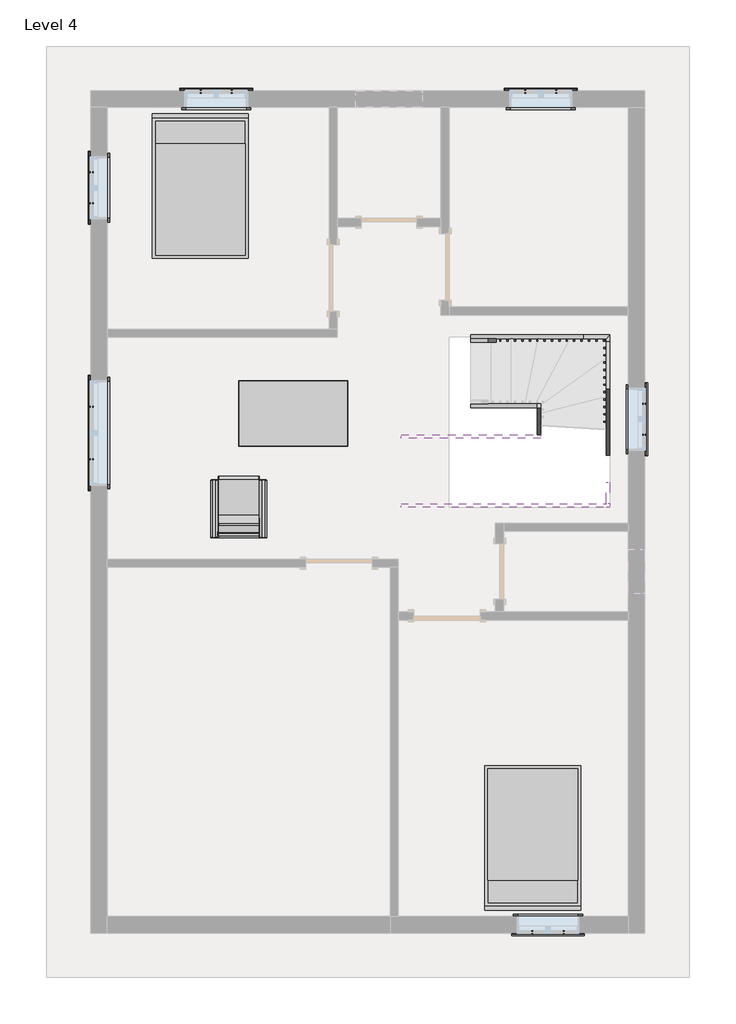
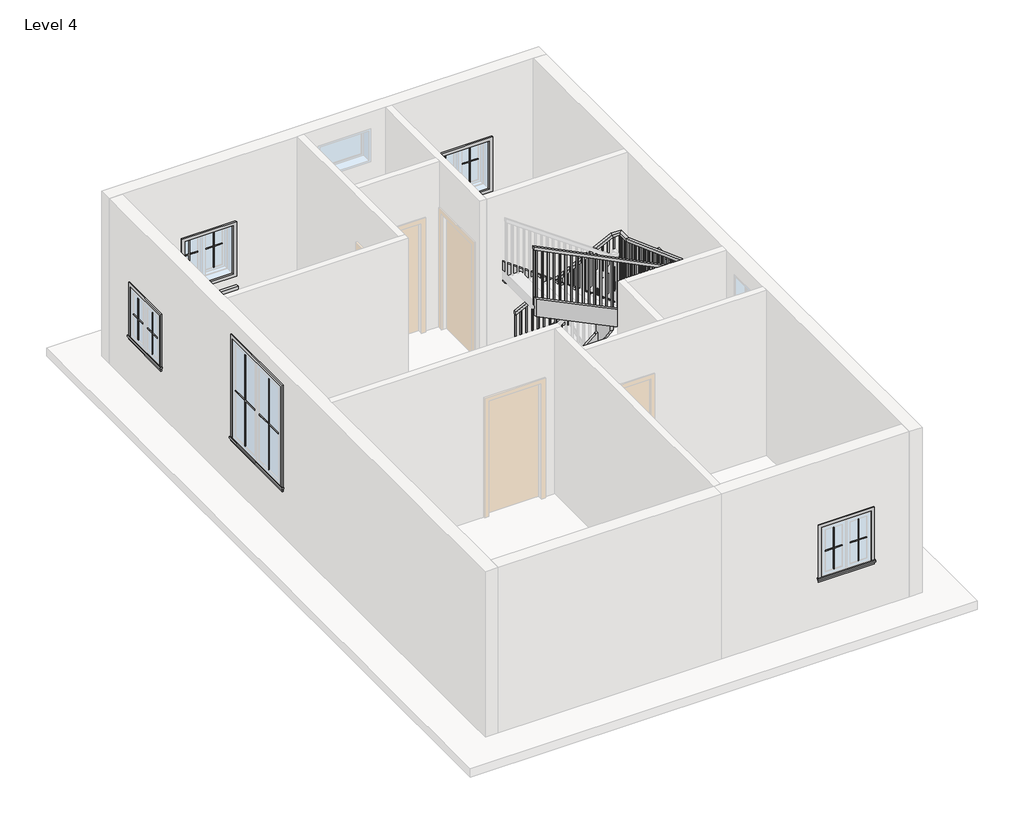
# One storey, part 2 of 2: 24 proxies, 9 members, 4 furniture elements, 1 railing.
"""IFC4 building model written with IfcOpenShell, lengths in millimetres."""

from ifc_helpers import new_model, si_unit, frame, origin, place, context, project, spatial, polyline, outline, extrude, faceted_brep, transform, mapped, element, save
from components import muntin_pattern_2x2_muntin_pattern_2x2_b3fe6957, muntin_pattern_2x2_muntin_pattern_2x2_3e0ecaf2, muntin_pattern_2x2_muntin_pattern_2x2_bff912c5, muntin_pattern_2x2_muntin_pattern_2x2_c2194282, trim_window_exterior_flat_with_sill_41619996, trim_window_exterior_flat_with_sill_e04b3088, trim_window_interior_flat_picture_frame_51c85655, trim_window_interior_flat_picture_frame_2a7685fe, furniture_f28dd14e, furniture_402a1f5e, bed_17739_bed_17739_15c61121, dining_table_14755_dining_table_14755_d89cb775

model = new_model("IFC4")

# Units and contexts
model_context = context("Model", 3, world=origin())
ifc_project = project(units=[si_unit("LENGTHUNIT", "METRE", prefix="MILLI")], contexts=[model_context])

# Site, building, storey
site = spatial("IfcSite", under=ifc_project)
building = spatial("IfcBuilding", under=site)
storey = spatial("IfcBuildingStorey", under=building, Name="Level 4", Elevation=6400.8)

# Proxies
placement = place(None, origin())
muntin_pattern_2x2_muntin_pattern_2x2_shape = muntin_pattern_2x2_muntin_pattern_2x2_b3fe6957(model_context)
element("IfcBuildingElementProxy", 1, Name="Muntin Pattern_2x2 : Muntin Pattern_2x2", ObjectType="Muntin Pattern_2x2 : Muntin Pattern_2x2", at=placement, inside=storey, context=model_context, shape_type="MappedRepresentation", body=[
    mapped(muntin_pattern_2x2_muntin_pattern_2x2_shape, transform((-3555.5290084, 6319.8685985, 7385.05), x_axis=(1.0, 0.0, 0.0), y_axis=(0.0, 1.0, 0.0), z_axis=(0.0, 0.0, 1.0))),
])
element("IfcBuildingElementProxy", 2, Name="Muntin Pattern_2x2 : Muntin Pattern_2x2", ObjectType="Muntin Pattern_2x2 : Muntin Pattern_2x2", at=placement, inside=storey, context=model_context, shape_type="MappedRepresentation", body=[
    mapped(muntin_pattern_2x2_muntin_pattern_2x2_shape, transform((1435.5709916, -5243.4814015, 7385.05), x_axis=(-1.0, 0.0, 0.0), y_axis=(0.0, -1.0, 0.0), z_axis=(0.0, 0.0, 1.0))),
])
element("IfcBuildingElementProxy", 3, Name="Muntin Pattern_2x2 : Muntin Pattern_2x2", ObjectType="Muntin Pattern_2x2 : Muntin Pattern_2x2", at=placement, inside=storey, context=model_context, shape_type="MappedRepresentation", body=[
    mapped(muntin_pattern_2x2_muntin_pattern_2x2_shape, transform((2545.2334916, 2028.8560985, 7385.05), x_axis=(0.0, -1.0, 0.0), y_axis=(1.0, 0.0, 0.0), z_axis=(0.0, 0.0, 1.0))),
])
element("IfcBuildingElementProxy", 4, Name="Muntin Pattern_2x2 : Muntin Pattern_2x2", ObjectType="Muntin Pattern_2x2 : Muntin Pattern_2x2", at=placement, inside=storey, context=model_context, shape_type="MappedRepresentation", body=[
    mapped(muntin_pattern_2x2_muntin_pattern_2x2_shape, transform((908.5209916, 6319.8685985, 7385.05), x_axis=(1.0, 0.0, 0.0), y_axis=(0.0, 1.0, 0.0), z_axis=(0.0, 0.0, 1.0))),
])
element("IfcBuildingElementProxy", 5, Name="Muntin Pattern_2x2 : Muntin Pattern_2x2", ObjectType="Muntin Pattern_2x2 : Muntin Pattern_2x2", at=placement, inside=storey, context=model_context, shape_type="MappedRepresentation", body=[
    mapped(muntin_pattern_2x2_muntin_pattern_2x2_shape, transform((-5055.7165084, 4781.5810985, 7385.05), x_axis=(0.0, 1.0, 0.0), y_axis=(-1.0, 0.0, 0.0), z_axis=(0.0, 0.0, 1.0))),
])
muntin_pattern_2x2_muntin_pattern_2x2_2_shape = muntin_pattern_2x2_muntin_pattern_2x2_3e0ecaf2(model_context)
element("IfcBuildingElementProxy", 6, Name="Muntin Pattern_2x2 : Muntin Pattern_2x2", ObjectType="Muntin Pattern_2x2 : Muntin Pattern_2x2", at=placement, inside=storey, context=model_context, shape_type="MappedRepresentation", body=[
    mapped(muntin_pattern_2x2_muntin_pattern_2x2_2_shape, transform((-3126.9040084, 6319.8685985, 7385.05), x_axis=(-1.0, 0.0, 0.0), y_axis=(0.0, -1.0, 0.0), z_axis=(0.0, 0.0, 1.0))),
])
element("IfcBuildingElementProxy", 7, Name="Muntin Pattern_2x2 : Muntin Pattern_2x2", ObjectType="Muntin Pattern_2x2 : Muntin Pattern_2x2", at=placement, inside=storey, context=model_context, shape_type="MappedRepresentation", body=[
    mapped(muntin_pattern_2x2_muntin_pattern_2x2_2_shape, transform((1006.9459916, -5243.4814015, 7385.05), x_axis=(1.0, 0.0, 0.0), y_axis=(0.0, 1.0, 0.0), z_axis=(0.0, 0.0, 1.0))),
])
element("IfcBuildingElementProxy", 8, Name="Muntin Pattern_2x2 : Muntin Pattern_2x2", ObjectType="Muntin Pattern_2x2 : Muntin Pattern_2x2", at=placement, inside=storey, context=model_context, shape_type="MappedRepresentation", body=[
    mapped(muntin_pattern_2x2_muntin_pattern_2x2_2_shape, transform((2545.2334916, 1600.2310985, 7385.05), x_axis=(0.0, 1.0, 0.0), y_axis=(-1.0, 0.0, 0.0), z_axis=(0.0, 0.0, 1.0))),
])
element("IfcBuildingElementProxy", 9, Name="Muntin Pattern_2x2 : Muntin Pattern_2x2", ObjectType="Muntin Pattern_2x2 : Muntin Pattern_2x2", at=placement, inside=storey, context=model_context, shape_type="MappedRepresentation", body=[
    mapped(muntin_pattern_2x2_muntin_pattern_2x2_2_shape, transform((1337.1459916, 6319.8685985, 7385.05), x_axis=(-1.0, 0.0, 0.0), y_axis=(0.0, -1.0, 0.0), z_axis=(0.0, 0.0, 1.0))),
])
element("IfcBuildingElementProxy", 10, Name="Muntin Pattern_2x2 : Muntin Pattern_2x2", ObjectType="Muntin Pattern_2x2 : Muntin Pattern_2x2", at=placement, inside=storey, context=model_context, shape_type="MappedRepresentation", body=[
    mapped(muntin_pattern_2x2_muntin_pattern_2x2_2_shape, transform((-5055.7165084, 5210.2060985, 7385.05), x_axis=(0.0, -1.0, 0.0), y_axis=(1.0, 0.0, 0.0), z_axis=(0.0, 0.0, 1.0))),
])
muntin_pattern_2x2_muntin_pattern_2x2_3_shape = muntin_pattern_2x2_muntin_pattern_2x2_bff912c5(model_context)
element("IfcBuildingElementProxy", 11, Name="Muntin Pattern_2x2 : Muntin Pattern_2x2", ObjectType="Muntin Pattern_2x2 : Muntin Pattern_2x2", at=placement, inside=storey, context=model_context, shape_type="MappedRepresentation", body=[
    mapped(muntin_pattern_2x2_muntin_pattern_2x2_3_shape, transform((-5055.7165084, 1263.6810985, 7385.05), x_axis=(0.0, 1.0, 0.0), y_axis=(-1.0, 0.0, 0.0), z_axis=(0.0, 0.0, 1.0))),
])
muntin_pattern_2x2_muntin_pattern_2x2_4_shape = muntin_pattern_2x2_muntin_pattern_2x2_c2194282(model_context)
element("IfcBuildingElementProxy", 12, Name="Muntin Pattern_2x2 : Muntin Pattern_2x2", ObjectType="Muntin Pattern_2x2 : Muntin Pattern_2x2", at=placement, inside=storey, context=model_context, shape_type="MappedRepresentation", body=[
    mapped(muntin_pattern_2x2_muntin_pattern_2x2_4_shape, transform((-5055.7165084, 1984.4060985, 7385.05), x_axis=(0.0, -1.0, 0.0), y_axis=(1.0, 0.0, 0.0), z_axis=(0.0, 0.0, 1.0))),
])
trim_window_exterior_flat_with_sill_shape = trim_window_exterior_flat_with_sill_41619996(model_context)
element("IfcBuildingElementProxy", 13, Name="Trim-Window-Exterior-Flat : with Sill", ObjectType="Trim-Window-Exterior-Flat : with Sill", at=placement, inside=storey, context=model_context, shape_type="MappedRepresentation", body=[
    mapped(trim_window_exterior_flat_with_sill_shape, transform((-3341.2165084, 6329.3935985, 8229.6), x_axis=(-1.0, 0.0, 0.0), y_axis=(0.0, 0.0, 1.0), z_axis=(0.0, 1.0, 0.0))),
])
element("IfcBuildingElementProxy", 14, Name="Trim-Window-Exterior-Flat : with Sill", ObjectType="Trim-Window-Exterior-Flat : with Sill", at=placement, inside=storey, context=model_context, shape_type="MappedRepresentation", body=[
    mapped(trim_window_exterior_flat_with_sill_shape, transform((1221.2584916, -5253.0064015, 8229.6), x_axis=(1.0, 0.0, 0.0), y_axis=(0.0, 0.0, 1.0), z_axis=(0.0, -1.0, 0.0))),
])
element("IfcBuildingElementProxy", 15, Name="Trim-Window-Exterior-Flat : with Sill", ObjectType="Trim-Window-Exterior-Flat : with Sill", at=placement, inside=storey, context=model_context, shape_type="MappedRepresentation", body=[
    mapped(trim_window_exterior_flat_with_sill_shape, transform((2554.7584916, 1814.5435985, 8229.6), x_axis=(0.0, 1.0, 0.0), y_axis=(0.0, 0.0, 1.0), z_axis=(1.0, 0.0, 0.0))),
])
element("IfcBuildingElementProxy", 16, Name="Trim-Window-Exterior-Flat : with Sill", ObjectType="Trim-Window-Exterior-Flat : with Sill", at=placement, inside=storey, context=model_context, shape_type="MappedRepresentation", body=[
    mapped(trim_window_exterior_flat_with_sill_shape, transform((1122.8334916, 6329.3935985, 8229.6), x_axis=(-1.0, 0.0, 0.0), y_axis=(0.0, 0.0, 1.0), z_axis=(0.0, 1.0, 0.0))),
])
element("IfcBuildingElementProxy", 17, Name="Trim-Window-Exterior-Flat : with Sill", ObjectType="Trim-Window-Exterior-Flat : with Sill", at=placement, inside=storey, context=model_context, shape_type="MappedRepresentation", body=[
    mapped(trim_window_exterior_flat_with_sill_shape, transform((-5065.2415084, 4995.8935985, 8229.6), x_axis=(0.0, -1.0, 0.0), y_axis=(0.0, 0.0, 1.0), z_axis=(-1.0, 0.0, 0.0))),
])
trim_window_exterior_flat_with_sill_2_shape = trim_window_exterior_flat_with_sill_e04b3088(model_context)
element("IfcBuildingElementProxy", 18, Name="Trim-Window-Exterior-Flat : with Sill", ObjectType="Trim-Window-Exterior-Flat : with Sill", at=placement, inside=storey, context=model_context, shape_type="MappedRepresentation", body=[
    mapped(trim_window_exterior_flat_with_sill_2_shape, transform((-5065.2415084, 1624.0435985, 9144.0), x_axis=(0.0, -1.0, 0.0), y_axis=(0.0, 0.0, 1.0), z_axis=(-1.0, 0.0, 0.0))),
])
trim_window_interior_flat_picture_frame_shape = trim_window_interior_flat_picture_frame_51c85655(model_context)
element("IfcBuildingElementProxy", 19, Name="Trim-Window-Interior-Flat : Picture Frame", ObjectType="Trim-Window-Interior-Flat : Picture Frame", at=placement, inside=storey, context=model_context, shape_type="MappedRepresentation", body=[
    mapped(trim_window_interior_flat_picture_frame_shape, transform((-3341.2165084, 6100.7935985, 8229.6), x_axis=(1.0, 0.0, 0.0), y_axis=(0.0, 0.0, 1.0), z_axis=(0.0, -1.0, 0.0))),
])
element("IfcBuildingElementProxy", 20, Name="Trim-Window-Interior-Flat : Picture Frame", ObjectType="Trim-Window-Interior-Flat : Picture Frame", at=placement, inside=storey, context=model_context, shape_type="MappedRepresentation", body=[
    mapped(trim_window_interior_flat_picture_frame_shape, transform((1221.2584916, -5024.4064015, 8229.6), x_axis=(-1.0, 0.0, 0.0), y_axis=(0.0, 0.0, 1.0), z_axis=(0.0, 1.0, 0.0))),
])
element("IfcBuildingElementProxy", 21, Name="Trim-Window-Interior-Flat : Picture Frame", ObjectType="Trim-Window-Interior-Flat : Picture Frame", at=placement, inside=storey, context=model_context, shape_type="MappedRepresentation", body=[
    mapped(trim_window_interior_flat_picture_frame_shape, transform((2326.1584916, 1814.5435985, 8229.6), x_axis=(0.0, -1.0, 0.0), y_axis=(0.0, 0.0, 1.0), z_axis=(-1.0, 0.0, 0.0))),
])
element("IfcBuildingElementProxy", 22, Name="Trim-Window-Interior-Flat : Picture Frame", ObjectType="Trim-Window-Interior-Flat : Picture Frame", at=placement, inside=storey, context=model_context, shape_type="MappedRepresentation", body=[
    mapped(trim_window_interior_flat_picture_frame_shape, transform((1122.8334916, 6100.7935985, 8229.6), x_axis=(1.0, 0.0, 0.0), y_axis=(0.0, 0.0, 1.0), z_axis=(0.0, -1.0, 0.0))),
])
element("IfcBuildingElementProxy", 23, Name="Trim-Window-Interior-Flat : Picture Frame", ObjectType="Trim-Window-Interior-Flat : Picture Frame", at=placement, inside=storey, context=model_context, shape_type="MappedRepresentation", body=[
    mapped(trim_window_interior_flat_picture_frame_shape, transform((-4836.6415084, 4995.8935985, 8229.6), x_axis=(0.0, 1.0, 0.0), y_axis=(0.0, 0.0, 1.0), z_axis=(1.0, 0.0, 0.0))),
])
trim_window_interior_flat_picture_frame_2_shape = trim_window_interior_flat_picture_frame_2a7685fe(model_context)
element("IfcBuildingElementProxy", 24, Name="Trim-Window-Interior-Flat : Picture Frame", ObjectType="Trim-Window-Interior-Flat : Picture Frame", at=placement, inside=storey, context=model_context, shape_type="MappedRepresentation", body=[
    mapped(trim_window_interior_flat_picture_frame_2_shape, transform((-4836.6415084, 1624.0435985, 9144.0), x_axis=(0.0, 1.0, 0.0), y_axis=(0.0, 0.0, 1.0), z_axis=(1.0, 0.0, 0.0))),
])

# Furniture
furniture_shape = furniture_f28dd14e(model_context)
furniture_2_shape = furniture_402a1f5e(model_context)
element("IfcFurniture", 25, at=placement, inside=storey, context=model_context, shape_type="MappedRepresentation", body=[
    mapped(furniture_shape, transform((-3032.3877006, 981.9349825, 6400.8), x_axis=(-1.0, 0.0, 0.0), y_axis=(0.0, -1.0, 0.0), z_axis=(0.0, 0.0, 1.0))),
    mapped(furniture_2_shape, transform((-3032.3877006, 981.9349825, 6400.8), x_axis=(-1.0, 0.0, 0.0), y_axis=(0.0, -1.0, 0.0), z_axis=(0.0, 0.0, 1.0))),
])
bed_17739_bed_17739_shape = bed_17739_bed_17739_15c61121(model_context)
element("IfcFurniture", 26, ObjectType="Bed_17739 : Bed_17739", at=placement, inside=storey, context=model_context, shape_type="MappedRepresentation", body=[
    mapped(bed_17739_bed_17739_shape, transform((-3560.2915084, 4995.8935985, 6400.8), x_axis=(1.0, 0.0, 0.0), y_axis=(0.0, 1.0, 0.0), z_axis=(0.0, 0.0, 1.0))),
])
element("IfcFurniture", 27, ObjectType="Bed_17739 : Bed_17739", at=placement, inside=storey, context=model_context, shape_type="MappedRepresentation", body=[
    mapped(bed_17739_bed_17739_shape, transform((1011.7084916, -3919.5064015, 6400.8), x_axis=(-1.0, 0.0, 0.0), y_axis=(0.0, -1.0, 0.0), z_axis=(0.0, 0.0, 1.0))),
])
dining_table_14755_dining_table_14755_shape = dining_table_14755_dining_table_14755_d89cb775(model_context)
element("IfcFurniture", 28, ObjectType="Dining_table_14755 : Dining_table_14755", at=placement, inside=storey, context=model_context, shape_type="MappedRepresentation", body=[
    mapped(dining_table_14755_dining_table_14755_shape, transform((-3032.3877006, 1444.8879061, 6400.8), x_axis=(1.0, 0.0, 0.0), y_axis=(0.0, 1.0, 0.0), z_axis=(0.0, 0.0, 1.0))),
])

# Members
element("IfcMember", 29, ObjectType="Stringer - 2\" Width", at=placement, inside=storey, context=model_context, shape_type="SweptSolid", body=[
    extrude(outline(polyline([(6640.2504763, 158.6923968), (6400.8, 158.6923968), (6400.8, 366.2169505), (7027.0639814, 1705.9967367), (7363.5193197, 1705.9967367), (6640.2504763, 158.6923968)])), frame((0.0, 2922.8476133, 0.0), z_axis=(0.0, 1.0, 0.0), x_axis=(0.0, 0.0, 1.0)), (0.0, 0.0, 1.0), 50.8),
])
element("IfcMember", 30, ObjectType="Stringer - 2\" Width", at=placement, inside=storey, context=model_context, shape_type="SweptSolid", body=[
    extrude(outline(polyline([(1705.9967367, 2922.8476133), (1705.9967367, 2973.6476133), (2072.9441983, 2973.6476133), (2022.1441983, 2922.8476133), (1705.9967367, 2922.8476133)])), frame((0.0, 0.0, 7027.0639814), z_axis=(0.0, 0.0, 1.0), x_axis=(1.0, 0.0, 0.0)), (0.0, 0.0, 1.0), 336.4553383),
])
element("IfcMember", 31, ObjectType="Stringer - 2\" Width", at=placement, inside=storey, context=model_context, shape_type="SweptSolid", body=[
    extrude(outline(polyline([(2022.1441983, 2922.8476133), (2072.9441983, 2973.6476133), (2072.9441983, 2883.4348143), (2022.1441983, 2883.4348143), (2022.1441983, 2922.8476133)])), frame((0.0, 0.0, 7027.0639814), z_axis=(0.0, 0.0, 1.0), x_axis=(1.0, 0.0, 0.0)), (0.0, 0.0, 1.0), 336.4553383),
])
element("IfcMember", 32, ObjectType="Stringer - 2\" Width", at=placement, inside=storey, context=model_context, shape_type="SweptSolid", body=[
    extrude(outline(polyline([(2883.4348143, 7363.5193197), (2883.4348143, 7027.0639814), (947.0260734, 7736.4990218), (947.0260734, 8072.9543601), (2883.4348143, 7363.5193197)])), frame((2022.1441983, 0.0, 0.0), z_axis=(1.0, 0.0, 0.0), x_axis=(0.0, 1.0, 0.0)), (0.0, 0.0, 1.0), 50.8),
])
element("IfcMember", 33, ObjectType="Stringer - 2\" Width", at=placement, inside=storey, context=model_context, shape_type="SweptSolid", body=[
    extrude(outline(polyline([(2022.1441983, 947.0260734), (2072.9441983, 947.0260734), (2072.9441983, 652.4935985), (2022.1441983, 652.4935985), (2022.1441983, 947.0260734)])), frame((0.0, 0.0, 7742.1754285), z_axis=(0.0, 0.0, 1.0), x_axis=(1.0, 0.0, 0.0)), (0.0, 0.0, 1.0), 324.6119022),
])
element("IfcMember", 34, ObjectType="Stringer - 2\" Width", at=placement, inside=storey, context=model_context, shape_type="SweptSolid", body=[
    extrude(outline(polyline([(6575.2551137, 158.6923968), (6400.8, 158.6923968), (6400.8, 426.0767146), (6934.9870321, 1072.5901835), (7330.3706215, 1072.5901835), (6575.2551137, 158.6923968)])), frame((0.0, 1973.2935985, 0.0), z_axis=(0.0, 1.0, 0.0), x_axis=(0.0, 0.0, 1.0)), (0.0, 0.0, 1.0), 50.8),
])
element("IfcMember", 35, ObjectType="Stringer - 2\" Width", at=placement, inside=storey, context=model_context, shape_type="SweptSolid", body=[
    extrude(outline(polyline([(2024.0935985, 7533.696008), (2024.0935985, 7030.9724164), (1602.0476133, 7584.5407029), (1602.0476133, 8087.2642945), (2024.0935985, 7533.696008)])), frame((1072.5901835, 0.0, 0.0), z_axis=(1.0, 0.0, 0.0), x_axis=(0.0, 1.0, 0.0)), (0.0, 0.0, 1.0), 50.8),
])
element("IfcMember", 36, ObjectType="Stringer - 2\" Width", at=placement, inside=storey, context=model_context, shape_type="SweptSolid", body=[
    extrude(outline(polyline([(7762.9113348, 1123.3901835), (8139.8379401, 1123.3901835), (9537.9009734, -798.3242294), (9160.9743681, -798.3242294), (7762.9113348, 1123.3901835)])), frame((0.0, 1551.2476133, 0.0), z_axis=(0.0, 1.0, 0.0), x_axis=(0.0, 0.0, 1.0)), (0.0, 0.0, 1.0), 50.8),
])
element("IfcMember", 37, ObjectType="Stringer - 2\" Width", at=placement, inside=storey, context=model_context, shape_type="SweptSolid", body=[
    extrude(outline(polyline([(7761.9873308, 2072.9441983), (8042.0397747, 2072.9441983), (9440.7971818, -798.3242294), (9116.1852796, -798.3242294), (7761.9873308, 1981.4757528), (7761.9873308, 2072.9441983)])), frame((0.0, 601.6935985, 0.0), z_axis=(0.0, 1.0, 0.0), x_axis=(0.0, 0.0, 1.0)), (0.0, 0.0, 1.0), 50.8),
])

# Railing
element("IfcRailing", 38, ObjectType="Handrail - Rectangular", at=placement, inside=storey, context=model_context, shape_type="SolidModel", body=[
    faceted_brep([(158.6923968, 2922.8476133, 7484.5333333), (158.6923968, 2922.8476133, 7427.8325724), (158.6923968, 2872.0476133, 7427.8325724), (158.6923968, 2872.0476133, 7484.5333333), (1841.0143863, 2922.8476133, 8318.6084972), (1852.9161672, 2922.8476133, 8267.8084972), (1852.9161672, 2872.0476133, 8267.8084972), (1841.0143863, 2872.0476133, 8318.6084972), (2022.1441983, 2922.8476133, 8318.6084972), (2022.1441983, 2922.8476133, 8267.8084972), (1971.3441983, 2872.0476133, 8267.8084972), (1971.3441983, 2872.0476133, 8318.6084972), (2022.1441983, 2686.7050655, 8318.6084972), (2022.1441983, 2677.692274, 8267.8084972), (1971.3441983, 2677.692274, 8267.8084972), (1971.3441983, 2686.7050655, 8318.6084972), (2022.1441983, 796.951655, 9010.9505936), (2022.1441983, 787.9388635, 8960.1505936), (1971.3441983, 787.9388635, 8960.1505936), (1971.3441983, 796.951655, 9010.9505936), (2022.1441983, 652.4935985, 9010.9505936), (2022.1441983, 652.4935985, 8960.1505936), (1971.3441983, 703.2935985, 8960.1505936), (1971.3441983, 703.2935985, 9010.9505936), (1909.402346, 652.4935985, 9010.9505936), (1897.4228813, 652.4935985, 8960.1505936), (1897.4228813, 703.2935985, 8960.1505936), (1909.402346, 703.2935985, 9010.9505936), (-798.3242294, 652.4935985, 10363.2), (-798.3242294, 703.2935985, 10363.2), (-798.3242294, 703.2935985, 10306.4174077), (-798.3242294, 652.4935985, 10306.4174077)], [[[0, 1, 2, 3]], [[1, 0, 4, 5]], [[2, 1, 5, 6]], [[3, 2, 6, 7]], [[0, 3, 7, 4]], [[5, 4, 8, 9]], [[6, 5, 9, 10]], [[7, 6, 10, 11]], [[4, 7, 11, 8]], [[9, 8, 12, 13]], [[10, 9, 13, 14]], [[11, 10, 14, 15]], [[8, 11, 15, 12]], [[13, 12, 16, 17]], [[14, 13, 17, 18]], [[15, 14, 18, 19]], [[12, 15, 19, 16]], [[17, 16, 20, 21]], [[18, 17, 21, 22]], [[19, 18, 22, 23]], [[16, 19, 23, 20]], [[21, 20, 24, 25]], [[22, 21, 25, 26]], [[23, 22, 26, 27]], [[20, 23, 27, 24]], [[28, 29, 30, 31]], [[25, 24, 28, 31]], [[26, 25, 31, 30]], [[27, 26, 30, 29]], [[24, 27, 29, 28]]]),
    extrude(outline(polyline([(10285.2709318, -755.9808017), (9279.4666667, -755.9808017), (9279.4666667, -736.9308017), (10275.7572862, -736.9308017), (10285.2709318, -755.9808017)])), frame((0.0, 668.3685985, 0.0), z_axis=(0.0, 1.0, 0.0), x_axis=(0.0, 0.0, 1.0)), (0.0, 0.0, 1.0), 19.05),
    extrude(outline(polyline([(10234.5314883, -654.3808017), (9279.4666667, -654.3808017), (9279.4666667, -635.3308017), (10225.0178426, -635.3308017), (10234.5314883, -654.3808017)])), frame((0.0, 668.3685985, 0.0), z_axis=(0.0, 1.0, 0.0), x_axis=(0.0, 0.0, 1.0)), (0.0, 0.0, 1.0), 19.05),
    extrude(outline(polyline([(10183.7920447, -552.7808017), (9279.4666667, -552.7808017), (9279.4666667, -533.7308017), (10174.2783991, -533.7308017), (10183.7920447, -552.7808017)])), frame((0.0, 668.3685985, 0.0), z_axis=(0.0, 1.0, 0.0), x_axis=(0.0, 0.0, 1.0)), (0.0, 0.0, 1.0), 19.05),
    extrude(outline(polyline([(10133.0526012, -451.1808017), (9110.1333333, -451.1808017), (9110.1333333, -432.1308017), (10123.5389555, -432.1308017), (10133.0526012, -451.1808017)])), frame((0.0, 668.3685985, 0.0), z_axis=(0.0, 1.0, 0.0), x_axis=(0.0, 0.0, 1.0)), (0.0, 0.0, 1.0), 19.05),
    extrude(outline(polyline([(10082.3131577, -349.5808017), (9110.1333333, -349.5808017), (9110.1333333, -330.5308017), (10072.799512, -330.5308017), (10082.3131577, -349.5808017)])), frame((0.0, 668.3685985, 0.0), z_axis=(0.0, 1.0, 0.0), x_axis=(0.0, 0.0, 1.0)), (0.0, 0.0, 1.0), 19.05),
    extrude(outline(polyline([(10031.5737141, -247.9808017), (8940.8, -247.9808017), (8940.8, -228.9308017), (10022.0600685, -228.9308017), (10031.5737141, -247.9808017)])), frame((0.0, 668.3685985, 0.0), z_axis=(0.0, 1.0, 0.0), x_axis=(0.0, 0.0, 1.0)), (0.0, 0.0, 1.0), 19.05),
    extrude(outline(polyline([(9980.8342706, -146.3808017), (8940.8, -146.3808017), (8940.8, -127.3308017), (9971.3206249, -127.3308017), (9980.8342706, -146.3808017)])), frame((0.0, 668.3685985, 0.0), z_axis=(0.0, 1.0, 0.0), x_axis=(0.0, 0.0, 1.0)), (0.0, 0.0, 1.0), 19.05),
    extrude(outline(polyline([(9930.094827, -44.7808017), (8940.8, -44.7808017), (8940.8, -25.7308017), (9920.5811814, -25.7308017), (9930.094827, -44.7808017)])), frame((0.0, 668.3685985, 0.0), z_axis=(0.0, 1.0, 0.0), x_axis=(0.0, 0.0, 1.0)), (0.0, 0.0, 1.0), 19.05),
    extrude(outline(polyline([(9879.3553835, 56.8191983), (8771.4666667, 56.8191983), (8771.4666667, 75.8691983), (9869.8417378, 75.8691983), (9879.3553835, 56.8191983)])), frame((0.0, 668.3685985, 0.0), z_axis=(0.0, 1.0, 0.0), x_axis=(0.0, 0.0, 1.0)), (0.0, 0.0, 1.0), 19.05),
    extrude(outline(polyline([(9828.61594, 158.4191983), (8771.4666667, 158.4191983), (8771.4666667, 177.4691983), (9819.1022943, 177.4691983), (9828.61594, 158.4191983)])), frame((0.0, 668.3685985, 0.0), z_axis=(0.0, 1.0, 0.0), x_axis=(0.0, 0.0, 1.0)), (0.0, 0.0, 1.0), 19.05),
    extrude(outline(polyline([(9777.8764964, 260.0191983), (8771.4666667, 260.0191983), (8771.4666667, 279.0691983), (9768.3628508, 279.0691983), (9777.8764964, 260.0191983)])), frame((0.0, 668.3685985, 0.0), z_axis=(0.0, 1.0, 0.0), x_axis=(0.0, 0.0, 1.0)), (0.0, 0.0, 1.0), 19.05),
    extrude(outline(polyline([(9727.1370529, 361.6191983), (8602.1333333, 361.6191983), (8602.1333333, 380.6691983), (9717.6234072, 380.6691983), (9727.1370529, 361.6191983)])), frame((0.0, 668.3685985, 0.0), z_axis=(0.0, 1.0, 0.0), x_axis=(0.0, 0.0, 1.0)), (0.0, 0.0, 1.0), 19.05),
    extrude(outline(polyline([(9676.3976093, 463.2191983), (8602.1333333, 463.2191983), (8602.1333333, 482.2691983), (9666.8839637, 482.2691983), (9676.3976093, 463.2191983)])), frame((0.0, 668.3685985, 0.0), z_axis=(0.0, 1.0, 0.0), x_axis=(0.0, 0.0, 1.0)), (0.0, 0.0, 1.0), 19.05),
    extrude(outline(polyline([(9625.6581658, 564.8191983), (8602.1333333, 564.8191983), (8602.1333333, 583.8691983), (9616.1445201, 583.8691983), (9625.6581658, 564.8191983)])), frame((0.0, 668.3685985, 0.0), z_axis=(0.0, 1.0, 0.0), x_axis=(0.0, 0.0, 1.0)), (0.0, 0.0, 1.0), 19.05),
    extrude(outline(polyline([(9574.9187223, 666.4191983), (8432.8, 666.4191983), (8432.8, 685.4691983), (9565.4050766, 685.4691983), (9574.9187223, 666.4191983)])), frame((0.0, 668.3685985, 0.0), z_axis=(0.0, 1.0, 0.0), x_axis=(0.0, 0.0, 1.0)), (0.0, 0.0, 1.0), 19.05),
    extrude(outline(polyline([(9524.1792787, 768.0191983), (8432.8, 768.0191983), (8432.8, 787.0691983), (9514.665633, 787.0691983), (9524.1792787, 768.0191983)])), frame((0.0, 668.3685985, 0.0), z_axis=(0.0, 1.0, 0.0), x_axis=(0.0, 0.0, 1.0)), (0.0, 0.0, 1.0), 19.05),
    extrude(outline(polyline([(9473.4398352, 869.6191983), (8432.8, 869.6191983), (8432.8, 888.6691983), (9463.9261895, 888.6691983), (9473.4398352, 869.6191983)])), frame((0.0, 668.3685985, 0.0), z_axis=(0.0, 1.0, 0.0), x_axis=(0.0, 0.0, 1.0)), (0.0, 0.0, 1.0), 19.05),
    extrude(outline(polyline([(9422.7003916, 971.2191983), (8432.8, 971.2191983), (8432.8, 990.2691983), (9413.186746, 990.2691983), (9422.7003916, 971.2191983)])), frame((0.0, 668.3685985, 0.0), z_axis=(0.0, 1.0, 0.0), x_axis=(0.0, 0.0, 1.0)), (0.0, 0.0, 1.0), 19.05),
    extrude(outline(polyline([(9371.9609481, 1072.8191983), (8263.4666667, 1072.8191983), (8263.4666667, 1091.8691983), (9362.4473024, 1091.8691983), (9371.9609481, 1072.8191983)])), frame((0.0, 668.3685985, 0.0), z_axis=(0.0, 1.0, 0.0), x_axis=(0.0, 0.0, 1.0)), (0.0, 0.0, 1.0), 19.05),
    extrude(outline(polyline([(9321.2215046, 1174.4191983), (8263.4666667, 1174.4191983), (8263.4666667, 1193.4691983), (9311.7078589, 1193.4691983), (9321.2215046, 1174.4191983)])), frame((0.0, 668.3685985, 0.0), z_axis=(0.0, 1.0, 0.0), x_axis=(0.0, 0.0, 1.0)), (0.0, 0.0, 1.0), 19.05),
    extrude(outline(polyline([(9270.482061, 1276.0191983), (8263.4666667, 1276.0191983), (8263.4666667, 1295.0691983), (9260.9684153, 1295.0691983), (9270.482061, 1276.0191983)])), frame((0.0, 668.3685985, 0.0), z_axis=(0.0, 1.0, 0.0), x_axis=(0.0, 0.0, 1.0)), (0.0, 0.0, 1.0), 19.05),
    extrude(outline(polyline([(9219.7426175, 1377.6191983), (8094.1333333, 1377.6191983), (8094.1333333, 1396.6691983), (9210.2289718, 1396.6691983), (9219.7426175, 1377.6191983)])), frame((0.0, 668.3685985, 0.0), z_axis=(0.0, 1.0, 0.0), x_axis=(0.0, 0.0, 1.0)), (0.0, 0.0, 1.0), 19.05),
    extrude(outline(polyline([(9169.0031739, 1479.2191983), (8094.1333333, 1479.2191983), (8094.1333333, 1498.2691983), (9159.4895283, 1498.2691983), (9169.0031739, 1479.2191983)])), frame((0.0, 668.3685985, 0.0), z_axis=(0.0, 1.0, 0.0), x_axis=(0.0, 0.0, 1.0)), (0.0, 0.0, 1.0), 19.05),
    extrude(outline(polyline([(9118.2637304, 1580.8191983), (8094.1333333, 1580.8191983), (8094.1333333, 1599.8691983), (9108.7500847, 1599.8691983), (9118.2637304, 1580.8191983)])), frame((0.0, 668.3685985, 0.0), z_axis=(0.0, 1.0, 0.0), x_axis=(0.0, 0.0, 1.0)), (0.0, 0.0, 1.0), 19.05),
    extrude(outline(polyline([(9067.5242869, 1682.4191983), (8094.1333333, 1682.4191983), (8094.1333333, 1701.4691983), (9058.0106412, 1701.4691983), (9067.5242869, 1682.4191983)])), frame((0.0, 668.3685985, 0.0), z_axis=(0.0, 1.0, 0.0), x_axis=(0.0, 0.0, 1.0)), (0.0, 0.0, 1.0), 19.05),
    extrude(outline(polyline([(9016.7848433, 1784.0191983), (8094.1333333, 1784.0191983), (8094.1333333, 1803.0691983), (9007.2711976, 1803.0691983), (9016.7848433, 1784.0191983)])), frame((0.0, 668.3685985, 0.0), z_axis=(0.0, 1.0, 0.0), x_axis=(0.0, 0.0, 1.0)), (0.0, 0.0, 1.0), 19.05),
    extrude(outline(polyline([(8966.0453998, 1885.6191983), (7924.8, 1885.6191983), (7924.8, 1904.6691983), (8956.5317541, 1904.6691983), (8966.0453998, 1885.6191983)])), frame((0.0, 668.3685985, 0.0), z_axis=(0.0, 1.0, 0.0), x_axis=(0.0, 0.0, 1.0)), (0.0, 0.0, 1.0), 19.05),
    extrude(outline(polyline([(2006.2691983, 773.3726133), (2006.2691983, 754.3226133), (1987.2191983, 754.3226133), (1987.2191983, 773.3726133), (2006.2691983, 773.3726133)])), frame((0.0, 0.0, 7924.8), z_axis=(0.0, 0.0, 1.0), x_axis=(1.0, 0.0, 0.0)), (0.0, 0.0, 1.0), 1035.3505936),
    extrude(outline(polyline([(874.9726133, 8928.2643546), (874.9726133, 7924.8), (855.9226133, 7924.8), (855.9226133, 8935.243634), (874.9726133, 8928.2643546)])), frame((1987.2191983, 0.0, 0.0), z_axis=(1.0, 0.0, 0.0), x_axis=(0.0, 1.0, 0.0)), (0.0, 0.0, 1.0), 19.05),
    extrude(outline(polyline([(976.5726133, 8891.0415315), (976.5726133, 7924.8), (957.5226133, 7924.8), (957.5226133, 8898.0208108), (976.5726133, 8891.0415315)])), frame((1987.2191983, 0.0, 0.0), z_axis=(1.0, 0.0, 0.0), x_axis=(0.0, 1.0, 0.0)), (0.0, 0.0, 1.0), 19.05),
    extrude(outline(polyline([(1078.1726133, 8853.8187083), (1078.1726133, 7924.8), (1059.1226133, 7924.8), (1059.1226133, 8860.7979877), (1078.1726133, 8853.8187083)])), frame((1987.2191983, 0.0, 0.0), z_axis=(1.0, 0.0, 0.0), x_axis=(0.0, 1.0, 0.0)), (0.0, 0.0, 1.0), 19.05),
    extrude(outline(polyline([(1179.7726133, 8816.5958852), (1179.7726133, 7924.8), (1160.7226133, 7924.8), (1160.7226133, 8823.5751645), (1179.7726133, 8816.5958852)])), frame((1987.2191983, 0.0, 0.0), z_axis=(1.0, 0.0, 0.0), x_axis=(0.0, 1.0, 0.0)), (0.0, 0.0, 1.0), 19.05),
    extrude(outline(polyline([(1281.3726133, 8779.373062), (1281.3726133, 7924.8), (1262.3226133, 7924.8), (1262.3226133, 8786.3523414), (1281.3726133, 8779.373062)])), frame((1987.2191983, 0.0, 0.0), z_axis=(1.0, 0.0, 0.0), x_axis=(0.0, 1.0, 0.0)), (0.0, 0.0, 1.0), 19.05),
    extrude(outline(polyline([(1382.9726133, 8742.1502389), (1382.9726133, 7755.4666667), (1363.9226133, 7755.4666667), (1363.9226133, 8749.1295182), (1382.9726133, 8742.1502389)])), frame((1987.2191983, 0.0, 0.0), z_axis=(1.0, 0.0, 0.0), x_axis=(0.0, 1.0, 0.0)), (0.0, 0.0, 1.0), 19.05),
    extrude(outline(polyline([(1484.5726133, 8704.9274157), (1484.5726133, 7755.4666667), (1465.5226133, 7755.4666667), (1465.5226133, 8711.9066951), (1484.5726133, 8704.9274157)])), frame((1987.2191983, 0.0, 0.0), z_axis=(1.0, 0.0, 0.0), x_axis=(0.0, 1.0, 0.0)), (0.0, 0.0, 1.0), 19.05),
    extrude(outline(polyline([(1586.1726133, 8667.7045926), (1586.1726133, 7755.4666667), (1567.1226133, 7755.4666667), (1567.1226133, 8674.6838719), (1586.1726133, 8667.7045926)])), frame((1987.2191983, 0.0, 0.0), z_axis=(1.0, 0.0, 0.0), x_axis=(0.0, 1.0, 0.0)), (0.0, 0.0, 1.0), 19.05),
    extrude(outline(polyline([(1687.7726133, 8630.4817694), (1687.7726133, 7755.4666667), (1668.7226133, 7755.4666667), (1668.7226133, 8637.4610488), (1687.7726133, 8630.4817694)])), frame((1987.2191983, 0.0, 0.0), z_axis=(1.0, 0.0, 0.0), x_axis=(0.0, 1.0, 0.0)), (0.0, 0.0, 1.0), 19.05),
    extrude(outline(polyline([(1789.3726133, 8593.2589463), (1789.3726133, 7586.1333333), (1770.3226133, 7586.1333333), (1770.3226133, 8600.2382256), (1789.3726133, 8593.2589463)])), frame((1987.2191983, 0.0, 0.0), z_axis=(1.0, 0.0, 0.0), x_axis=(0.0, 1.0, 0.0)), (0.0, 0.0, 1.0), 19.05),
    extrude(outline(polyline([(1890.9726133, 8556.0361231), (1890.9726133, 7586.1333333), (1871.9226133, 7586.1333333), (1871.9226133, 8563.0154025), (1890.9726133, 8556.0361231)])), frame((1987.2191983, 0.0, 0.0), z_axis=(1.0, 0.0, 0.0), x_axis=(0.0, 1.0, 0.0)), (0.0, 0.0, 1.0), 19.05),
    extrude(outline(polyline([(1992.5726133, 8518.8133), (1992.5726133, 7586.1333333), (1973.5226133, 7586.1333333), (1973.5226133, 8525.7925793), (1992.5726133, 8518.8133)])), frame((1987.2191983, 0.0, 0.0), z_axis=(1.0, 0.0, 0.0), x_axis=(0.0, 1.0, 0.0)), (0.0, 0.0, 1.0), 19.05),
    extrude(outline(polyline([(2094.1726133, 8481.5904769), (2094.1726133, 7586.1333333), (2075.1226133, 7586.1333333), (2075.1226133, 8488.5697562), (2094.1726133, 8481.5904769)])), frame((1987.2191983, 0.0, 0.0), z_axis=(1.0, 0.0, 0.0), x_axis=(0.0, 1.0, 0.0)), (0.0, 0.0, 1.0), 19.05),
    extrude(outline(polyline([(2195.7726133, 8444.3676537), (2195.7726133, 7416.8), (2176.7226133, 7416.8), (2176.7226133, 8451.346933), (2195.7726133, 8444.3676537)])), frame((1987.2191983, 0.0, 0.0), z_axis=(1.0, 0.0, 0.0), x_axis=(0.0, 1.0, 0.0)), (0.0, 0.0, 1.0), 19.05),
    extrude(outline(polyline([(2297.3726133, 8407.1448306), (2297.3726133, 7416.8), (2278.3226133, 7416.8), (2278.3226133, 8414.1241099), (2297.3726133, 8407.1448306)])), frame((1987.2191983, 0.0, 0.0), z_axis=(1.0, 0.0, 0.0), x_axis=(0.0, 1.0, 0.0)), (0.0, 0.0, 1.0), 19.05),
    extrude(outline(polyline([(2398.9726133, 8369.9220074), (2398.9726133, 7416.8), (2379.9226133, 7416.8), (2379.9226133, 8376.9012867), (2398.9726133, 8369.9220074)])), frame((1987.2191983, 0.0, 0.0), z_axis=(1.0, 0.0, 0.0), x_axis=(0.0, 1.0, 0.0)), (0.0, 0.0, 1.0), 19.05),
    extrude(outline(polyline([(2500.5726133, 8332.6991843), (2500.5726133, 7416.8), (2481.5226133, 7416.8), (2481.5226133, 8339.6784636), (2500.5726133, 8332.6991843)])), frame((1987.2191983, 0.0, 0.0), z_axis=(1.0, 0.0, 0.0), x_axis=(0.0, 1.0, 0.0)), (0.0, 0.0, 1.0), 19.05),
    extrude(outline(polyline([(2602.1726133, 8295.4763611), (2602.1726133, 7416.8), (2583.1226133, 7416.8), (2583.1226133, 8302.4556405), (2602.1726133, 8295.4763611)])), frame((1987.2191983, 0.0, 0.0), z_axis=(1.0, 0.0, 0.0), x_axis=(0.0, 1.0, 0.0)), (0.0, 0.0, 1.0), 19.05),
    extrude(outline(polyline([(2006.2691983, 2703.7726133), (2006.2691983, 2684.7226133), (1987.2191983, 2684.7226133), (1987.2191983, 2703.7726133), (2006.2691983, 2703.7726133)])), frame((0.0, 0.0, 7247.4666667), z_axis=(0.0, 0.0, 1.0), x_axis=(1.0, 0.0, 0.0)), (0.0, 0.0, 1.0), 1020.3418305),
    extrude(outline(polyline([(2006.2691983, 2805.3726133), (2006.2691983, 2786.3226133), (1987.2191983, 2786.3226133), (1987.2191983, 2805.3726133), (2006.2691983, 2805.3726133)])), frame((0.0, 0.0, 7247.4666667), z_axis=(0.0, 0.0, 1.0), x_axis=(1.0, 0.0, 0.0)), (0.0, 0.0, 1.0), 1020.3418305),
    extrude(outline(polyline([(1977.9673968, 2906.9726133), (1997.0173968, 2906.9726133), (1997.0173968, 2887.9226133), (1977.9673968, 2887.9226133), (1977.9673968, 2906.9726133)])), frame((0.0, 0.0, 7247.4666667), z_axis=(0.0, 0.0, 1.0), x_axis=(1.0, 0.0, 0.0)), (0.0, 0.0, 1.0), 1020.3418305),
    extrude(outline(polyline([(1876.3673968, 2906.9726133), (1895.4173968, 2906.9726133), (1895.4173968, 2887.9226133), (1876.3673968, 2887.9226133), (1876.3673968, 2906.9726133)])), frame((0.0, 0.0, 7247.4666667), z_axis=(0.0, 0.0, 1.0), x_axis=(1.0, 0.0, 0.0)), (0.0, 0.0, 1.0), 1020.3418305),
    extrude(outline(polyline([(8229.0632695, 1774.7673968), (7247.4666667, 1774.7673968), (7247.4666667, 1793.8173968), (8238.5080321, 1793.8173968), (8229.0632695, 1774.7673968)])), frame((0.0, 2887.9226133, 0.0), z_axis=(0.0, 1.0, 0.0), x_axis=(0.0, 0.0, 1.0)), (0.0, 0.0, 1.0), 19.05),
    extrude(outline(polyline([(8178.6912021, 1673.1673968), (7247.4666667, 1673.1673968), (7247.4666667, 1692.2173968), (8188.1359647, 1692.2173968), (8178.6912021, 1673.1673968)])), frame((0.0, 2887.9226133, 0.0), z_axis=(0.0, 1.0, 0.0), x_axis=(0.0, 0.0, 1.0)), (0.0, 0.0, 1.0), 19.05),
    extrude(outline(polyline([(8128.3191347, 1571.5673968), (7247.4666667, 1571.5673968), (7247.4666667, 1590.6173968), (8137.7638973, 1590.6173968), (8128.3191347, 1571.5673968)])), frame((0.0, 2887.9226133, 0.0), z_axis=(0.0, 1.0, 0.0), x_axis=(0.0, 0.0, 1.0)), (0.0, 0.0, 1.0), 19.05),
    extrude(outline(polyline([(8077.9470673, 1469.9673968), (7078.1333333, 1469.9673968), (7078.1333333, 1489.0173968), (8087.3918299, 1489.0173968), (8077.9470673, 1469.9673968)])), frame((0.0, 2887.9226133, 0.0), z_axis=(0.0, 1.0, 0.0), x_axis=(0.0, 0.0, 1.0)), (0.0, 0.0, 1.0), 19.05),
    extrude(outline(polyline([(8027.5749999, 1368.3673968), (7078.1333333, 1368.3673968), (7078.1333333, 1387.4173968), (8037.0197625, 1387.4173968), (8027.5749999, 1368.3673968)])), frame((0.0, 2887.9226133, 0.0), z_axis=(0.0, 1.0, 0.0), x_axis=(0.0, 0.0, 1.0)), (0.0, 0.0, 1.0), 19.05),
    extrude(outline(polyline([(7977.2029325, 1266.7673968), (7078.1333333, 1266.7673968), (7078.1333333, 1285.8173968), (7986.6476951, 1285.8173968), (7977.2029325, 1266.7673968)])), frame((0.0, 2887.9226133, 0.0), z_axis=(0.0, 1.0, 0.0), x_axis=(0.0, 0.0, 1.0)), (0.0, 0.0, 1.0), 19.05),
    extrude(outline(polyline([(7926.8308651, 1165.1673968), (7078.1333333, 1165.1673968), (7078.1333333, 1184.2173968), (7936.2756277, 1184.2173968), (7926.8308651, 1165.1673968)])), frame((0.0, 2887.9226133, 0.0), z_axis=(0.0, 1.0, 0.0), x_axis=(0.0, 0.0, 1.0)), (0.0, 0.0, 1.0), 19.05),
    extrude(outline(polyline([(7876.4587977, 1063.5673968), (6908.8, 1063.5673968), (6908.8, 1082.6173968), (7885.9035603, 1082.6173968), (7876.4587977, 1063.5673968)])), frame((0.0, 2887.9226133, 0.0), z_axis=(0.0, 1.0, 0.0), x_axis=(0.0, 0.0, 1.0)), (0.0, 0.0, 1.0), 19.05),
    extrude(outline(polyline([(7826.0867303, 961.9673968), (6908.8, 961.9673968), (6908.8, 981.0173968), (7835.5314929, 981.0173968), (7826.0867303, 961.9673968)])), frame((0.0, 2887.9226133, 0.0), z_axis=(0.0, 1.0, 0.0), x_axis=(0.0, 0.0, 1.0)), (0.0, 0.0, 1.0), 19.05),
    extrude(outline(polyline([(7775.7146629, 860.3673968), (6908.8, 860.3673968), (6908.8, 879.4173968), (7785.1594255, 879.4173968), (7775.7146629, 860.3673968)])), frame((0.0, 2887.9226133, 0.0), z_axis=(0.0, 1.0, 0.0), x_axis=(0.0, 0.0, 1.0)), (0.0, 0.0, 1.0), 19.05),
    extrude(outline(polyline([(7725.3425955, 758.7673968), (6908.8, 758.7673968), (6908.8, 777.8173968), (7734.7873581, 777.8173968), (7725.3425955, 758.7673968)])), frame((0.0, 2887.9226133, 0.0), z_axis=(0.0, 1.0, 0.0), x_axis=(0.0, 0.0, 1.0)), (0.0, 0.0, 1.0), 19.05),
    extrude(outline(polyline([(7674.9705281, 657.1673968), (6739.4666667, 657.1673968), (6739.4666667, 676.2173968), (7684.4152907, 676.2173968), (7674.9705281, 657.1673968)])), frame((0.0, 2887.9226133, 0.0), z_axis=(0.0, 1.0, 0.0), x_axis=(0.0, 0.0, 1.0)), (0.0, 0.0, 1.0), 19.05),
    extrude(outline(polyline([(7624.5984607, 555.5673968), (6739.4666667, 555.5673968), (6739.4666667, 574.6173968), (7634.0432233, 574.6173968), (7624.5984607, 555.5673968)])), frame((0.0, 2887.9226133, 0.0), z_axis=(0.0, 1.0, 0.0), x_axis=(0.0, 0.0, 1.0)), (0.0, 0.0, 1.0), 19.05),
    extrude(outline(polyline([(7574.2263933, 453.9673968), (6739.4666667, 453.9673968), (6739.4666667, 473.0173968), (7583.6711559, 473.0173968), (7574.2263933, 453.9673968)])), frame((0.0, 2887.9226133, 0.0), z_axis=(0.0, 1.0, 0.0), x_axis=(0.0, 0.0, 1.0)), (0.0, 0.0, 1.0), 19.05),
    extrude(outline(polyline([(7523.8543259, 352.3673968), (6570.1333333, 352.3673968), (6570.1333333, 371.4173968), (7533.2990885, 371.4173968), (7523.8543259, 352.3673968)])), frame((0.0, 2887.9226133, 0.0), z_axis=(0.0, 1.0, 0.0), x_axis=(0.0, 0.0, 1.0)), (0.0, 0.0, 1.0), 19.05),
    extrude(outline(polyline([(7473.4822585, 250.7673968), (6570.1333333, 250.7673968), (6570.1333333, 269.8173968), (7482.9270211, 269.8173968), (7473.4822585, 250.7673968)])), frame((0.0, 2887.9226133, 0.0), z_axis=(0.0, 1.0, 0.0), x_axis=(0.0, 0.0, 1.0)), (0.0, 0.0, 1.0), 19.05),
    extrude(outline(polyline([(2006.2691983, 687.4185985), (2006.2691983, 668.3685985), (1987.2191983, 668.3685985), (1987.2191983, 687.4185985), (2006.2691983, 687.4185985)])), frame((0.0, 0.0, 7924.8), z_axis=(0.0, 0.0, 1.0), x_axis=(1.0, 0.0, 0.0)), (0.0, 0.0, 1.0), 1035.3505936),
    extrude(outline(polyline([(1987.2191983, 2906.9726133), (2006.2691983, 2906.9726133), (2006.2691983, 2887.9226133), (1987.2191983, 2887.9226133), (1987.2191983, 2906.9726133)])), frame((0.0, 0.0, 7247.4666667), z_axis=(0.0, 0.0, 1.0), x_axis=(1.0, 0.0, 0.0)), (0.0, 0.0, 1.0), 1020.3418305),
    extrude(outline(polyline([(10306.4174077, -798.3242294), (9279.4666667, -798.3242294), (9279.4666667, -779.2742294), (10296.9037621, -779.2742294), (10306.4174077, -798.3242294)])), frame((0.0, 668.3685985, 0.0), z_axis=(0.0, 1.0, 0.0), x_axis=(0.0, 0.0, 1.0)), (0.0, 0.0, 1.0), 19.05),
    extrude(outline(polyline([(7427.8325724, 158.6923968), (6570.1333333, 158.6923968), (6570.1333333, 177.7423968), (7437.277335, 177.7423968), (7427.8325724, 158.6923968)])), frame((0.0, 2887.9226133, 0.0), z_axis=(0.0, 1.0, 0.0), x_axis=(0.0, 0.0, 1.0)), (0.0, 0.0, 1.0), 19.05),
])

save(model, "model.ifc")

# Revit data of these elements
# Type "Muntin Pattern_2x2 : Muntin Pattern_2x2"
#   Width [instance default] = 4' - 0"
#   Thickness = 0' - 0 1/2"
#   Height [instance default] = 4' - 0"
#   Distance = 0' - 0 3/4"
#   Interior Material [instance default] = none
#   Exterior Material [instance default] = none
#   Default Elevation = 0
# Type "Trim-Window-Exterior-Flat : with Sill"
#   Trim Width = 0' - 2 1/4"
#   Trim Thickness_Picture Frame = 0' - 1 1/4"
#   Trim Thickness_with Sill = 0' - 0 3/4"
#   Sill Thickness = 0' - 1 1/4"
#   Opening Width [instance default] = 2' - 0"
#   Opening Height [instance default] = 3' - 0"
#   Default Elevation = 4' - 0"
#   Sill = yes
#   Picture Frame = no
#   Trim Material [instance default] = none
# Type "Trim-Window-Interior-Flat : Picture Frame"
#   Trim Thickness_Picture Frame = 0' - 1 1/4"
#   Trim Width = 0' - 2 1/4"
#   Trim Thickness_with Sill = 0' - 0 3/4"
#   Sill Thickness = 0' - 1 1/4"
#   Opening Width [instance default] = 2' - 0"
#   Opening Height [instance default] = 3' - 0"
#   Default Elevation = 4' - 0"
#   Sill = no
#   Picture Frame = yes
#   Trim Material [instance default] = none
# Type
#   Width [instance] = 2' - 6.31496"
#   Default Elevation = 0
# Type "Bed_17739 : Bed_17739"
#   Default Elevation = 0
# Type "Dining_table_14755 : Dining_table_14755"
#   Lengte [instance default] = 4' - 11.05512"
#   Breedte [instance default] = 2' - 11.43307"
#   Tafelblad = none
#   Poten = none
#   Default Elevation = 0
# Type "Handrail - Rectangular"
#   Assembly Code = "C2010400"
#   built-in parameter 1008612 = 0.0416667 (stored number, unit not read)
#   built-in parameter 1008611 = 0.0416667 (stored number, unit not read)
#   built-in parameter 1008609 = 0.333333 (stored number, unit not read)
#   built-in parameter 1008604 = 0.166667 (stored number, unit not read)
#   built-in parameter 1008603 = 0.166667 (stored number, unit not read)
#   Railing Height = 3' - 0"
#   built-in parameter 1008630 = 2
#   built-in parameter 1008610 = 2
#   built-in parameter 1008618 = Baluster - Square : 3/4"
# Elements 1, 2, 3, 4, 5, 6, 7, 8, 9, 10 (IfcBuildingElementProxy, "Muntin Pattern_2x2 : Muntin Pattern_2x2")
#   Width = 0' - 11 5/8"
#   Height = 2' - 6 1/2"
#   Interior Material = Wood - Stained
#   Exterior Material = Clad - White
#   Phase Created = New Construction
#   Materials on its faces: "Clad - White", "Wood - Stained"
# Elements 11, 12 (IfcBuildingElementProxy, "Muntin Pattern_2x2 : Muntin Pattern_2x2")
#   Width = 1' - 11 1/8"
#   Height = 5' - 6 1/2"
#   Interior Material = Wood - Stained
#   Exterior Material = Clad - White
#   Phase Created = New Construction
#   Materials on its faces: "Clad - White", "Wood - Stained"
# Elements 13, 14, 15, 16, 17 (IfcBuildingElementProxy, "Trim-Window-Exterior-Flat : with Sill")
#   Opening Width = 2' - 10"
#   Opening Height = 3' - 0"
#   Trim Material = Clad - White
#   Phase Created = New Construction
#   Materials on its faces: "Clad - White"
# Element 18 (IfcBuildingElementProxy, "Trim-Window-Exterior-Flat : with Sill")
#   Opening Width = 4' - 9"
#   Opening Height = 6' - 0"
#   Trim Material = Clad - White
#   Phase Created = New Construction
#   Materials on its faces: "Clad - White"
# Elements 19, 20, 21, 22, 23 (IfcBuildingElementProxy, "Trim-Window-Interior-Flat : Picture Frame")
#   Opening Width = 2' - 10"
#   Opening Height = 3' - 0"
#   Trim Material = Wood - Stained
#   Phase Created = New Construction
#   Materials on its faces: "Wood - Stained"
# Element 24 (IfcBuildingElementProxy, "Trim-Window-Interior-Flat : Picture Frame")
#   Opening Width = 4' - 9"
#   Opening Height = 6' - 0"
#   Trim Material = Wood - Stained
#   Phase Created = New Construction
#   Materials on its faces: "Wood - Stained"
# Element 25 (IfcFurniture)
#   Width = 2' - 6.31496"
#   Phase Created = New Construction
# Elements 26, 27 (IfcFurniture, "Bed_17739 : Bed_17739")
#   Phase Created = New Construction
#   Materials on its faces: "legs", "sheets", "bed frame", "Blanket"
# Element 28 (IfcFurniture, "Dining_table_14755 : Dining_table_14755")
#   Lengte = 4' - 11.05512"
#   Breedte = 2' - 11.43307"
#   Phase Created = New Construction
# Elements 29, 30, 31, 32, 33, 34, 35, 36, 37 (IfcMember, "Stringer - 2\" Width")
#   Phase Created = New Construction
# Element 38 (IfcRailing, "Handrail - Rectangular")
#   Phase Created = New Construction
# Materials
#   "Clad - White": class "Wood", colour RGB 242 242 238, transparency 0, Cost = 0
#   "Wood - Stained": class "Wood", colour RGB 224 178 126, transparency 0, Cost = 0
#   "legs": colour RGB 90 73 37, transparency 0, Cost = 0
#   "sheets": colour RGB 200 195 176, transparency 0, Cost = 0
#   "bed frame": colour RGB 90 73 37, transparency 0, Cost = 0
#   "Blanket": class "System", colour RGB 59 0 1, transparency 0, Cost = 0
